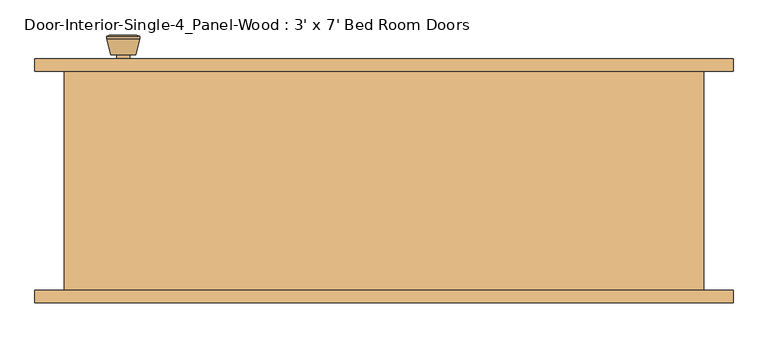
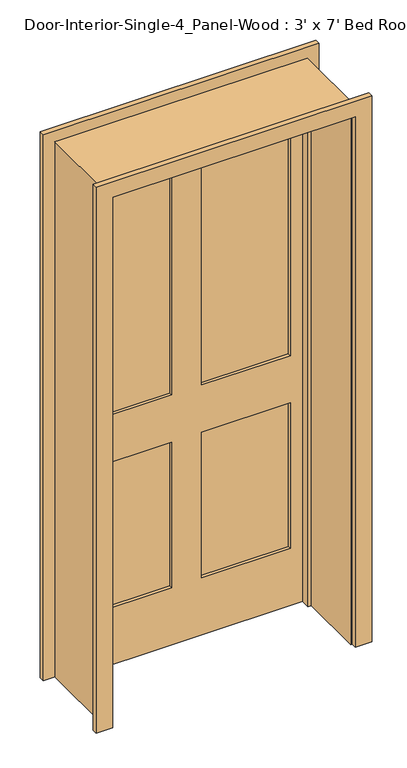
"""IFC4 building model written with IfcOpenShell, lengths in millimetres: door geometry, Door-Interior-Single-4_Panel-Wood : 3' x 7' Bed Room Doors."""

from ifc_helpers import new_model, si_unit, point, frame, frame_2d, origin, place, context, project, spatial, polyline, circle_curve, trimmed, segment, composite_curve, outline, extrude, faceted_brep, source, transform, mapped, element, save
from ifc_brep_helpers import plane_surface, cylinder_surface, revolved_surface, advanced_brep


def door_interior_single_4_panel_wood_3_x_7_bed_room_doors_791c550c(model_context):
    return source(origin(), model_context, "Body", "SolidModel", [
        advanced_brep(
        [(-393.7, 121.0, 914.4), (-383.7, 121.0, 914.4), (-403.7, 121.0, 914.4), (-373.2241324, 72.0, 914.4), (-393.7, 72.0, 914.4), (-414.1758676, 72.0, 914.4), (-368.7, 73.8278681, 914.4), (-418.7, 73.8278681, 914.4), (-368.7, 77.2915463, 914.4), (-418.7, 77.2915463, 914.4), (-375.063764, 102.0, 914.4), (-412.336236, 102.0, 914.4), (-383.7, 102.0, 914.4), (-403.7, 102.0, 914.4)],
        [
            (0, 1),
            (1, 2, circle_curve(frame((-393.7, 121.0, 914.4), z_axis=(0.0, 1.0, 0.0), x_axis=(-1.0, 0.0, 0.0)), 10.0)),
            (2, 0),
            (2, 1, circle_curve(frame((-393.7, 121.0, 914.4), z_axis=(0.0, 1.0, 0.0), x_axis=(-1.0, 0.0, 0.0)), 10.0)),
            (3, 4),
            (4, 5),
            (5, 3, circle_curve(frame((-393.7, 72.0, 914.4), z_axis=(0.0, -1.0, 0.0), x_axis=(-1.0, 0.0, 0.0)), 20.4758676)),
            (3, 5, circle_curve(frame((-393.7, 72.0, 914.4), z_axis=(0.0, -1.0, 0.0), x_axis=(-1.0, 0.0, 0.0)), 20.4758676)),
            (6, 3),
            (5, 7),
            (7, 6, circle_curve(frame((-393.7, 73.8278681, 914.4), z_axis=(0.0, -1.0, 0.0), x_axis=(-1.0, 0.0, 0.0)), 25.0)),
            (6, 7, circle_curve(frame((-393.7, 73.8278681, 914.4), z_axis=(0.0, -1.0, 0.0), x_axis=(-1.0, 0.0, 0.0)), 25.0)),
            (8, 6),
            (7, 9),
            (9, 8, circle_curve(frame((-393.7, 77.2915463, 914.4), z_axis=(0.0, -1.0, 0.0), x_axis=(-1.0, 0.0, 0.0)), 25.0)),
            (8, 9, circle_curve(frame((-393.7, 77.2915463, 914.4), z_axis=(0.0, -1.0, 0.0), x_axis=(-1.0, 0.0, 0.0)), 25.0)),
            (10, 8),
            (9, 11),
            (11, 10, circle_curve(frame((-393.7, 102.0, 914.4), z_axis=(0.0, -1.0, 0.0), x_axis=(-1.0, 0.0, 0.0)), 18.636236)),
            (10, 11, circle_curve(frame((-393.7, 102.0, 914.4), z_axis=(0.0, -1.0, 0.0), x_axis=(-1.0, 0.0, 0.0)), 18.636236)),
            (12, 10),
            (11, 13),
            (13, 12, circle_curve(frame((-393.7, 102.0, 914.4), z_axis=(0.0, -1.0, 0.0), x_axis=(-1.0, 0.0, 0.0)), 10.0)),
            (12, 13, circle_curve(frame((-393.7, 102.0, 914.4), z_axis=(0.0, -1.0, 0.0), x_axis=(-1.0, 0.0, 0.0)), 10.0)),
            (1, 12),
            (13, 2),
        ],
        [
            plane_surface(frame((-393.7, 121.0, 914.4), z_axis=(0.0, 1.0, 0.0), x_axis=(-1.0, 0.0, 0.0))),
            plane_surface(frame((-393.7, 72.0, 914.4), z_axis=(0.0, -1.0, 0.0), x_axis=(-1.0, 0.0, 0.0))),
            revolved_surface(polyline([(-414.1758676, 72.0, 914.4), (-418.7, 73.8278681, 914.4)]), (-393.7, 121.0, 914.4), (0.0, 1.0, 0.0)),
            cylinder_surface(frame((-393.7, 121.0, 914.4), z_axis=(0.0, 1.0, 0.0), x_axis=(-1.0, 0.0, 0.0)), 25.0),
            revolved_surface(polyline([(-418.7, 77.2915463, 914.4), (-412.336236, 102.0, 914.4)]), (-393.7, 121.0, 914.4), (0.0, 1.0, 0.0)),
            plane_surface(frame((-393.7, 102.0, 914.4), z_axis=(0.0, 1.0, 0.0), x_axis=(-1.0, 0.0, 0.0))),
            cylinder_surface(frame((-393.7, 121.0, 914.4), z_axis=(0.0, 1.0, 0.0), x_axis=(-1.0, 0.0, 0.0)), 10.0),
        ],
        [
            (0, [[1, 2, 3]]),
            (0, [[-3, 4, -1]]),
            (1, [[5, 6, 7]]),
            (1, [[-6, -5, 8]]),
            (2, [[9, -7, 10, 11]]),
            (2, [[-10, -8, -9, 12]]),
            (3, [[13, -11, 14, 15]]),
            (3, [[-14, -12, -13, 16]]),
            (4, [[17, -15, 18, 19]]),
            (4, [[-18, -16, -17, 20]]),
            (5, [[21, -19, 22, 23]]),
            (5, [[-22, -20, -21, 24]]),
            (6, [[25, -23, 26, -2]]),
            (6, [[-26, -24, -25, -4]]),
        ],
    ),
        extrude(outline(composite_curve([segment(trimmed(circle_curve(frame_2d((914.4, -393.7)), 30.0), [point((914.4, -423.7))], [point((914.4, -363.7))], False, "CARTESIAN"), True, "CONTINUOUS"), segment(trimmed(circle_curve(frame_2d((914.4, -393.7)), 30.0), [point((914.4, -363.7))], [point((914.4, -423.7))], False, "CARTESIAN"), True, "CONTINUOUS")], self_intersect=False)), frame((0.0, 121.0, 0.0), z_axis=(0.0, 1.0, 0.0), x_axis=(0.0, 0.0, 1.0)), (0.0, 0.0, 1.0), 6.0),
        advanced_brep(
        [(-393.7, 167.925, 914.4), (-403.7, 167.925, 914.4), (-383.7, 167.925, 914.4), (-373.2241324, 216.925, 914.4), (-414.1758676, 216.925, 914.4), (-393.7, 216.925, 914.4), (-368.7, 215.0971319, 914.4), (-418.7, 215.0971319, 914.4), (-368.7, 211.6334537, 914.4), (-418.7, 211.6334537, 914.4), (-375.063764, 186.925, 914.4), (-412.336236, 186.925, 914.4), (-383.7, 186.925, 914.4), (-403.7, 186.925, 914.4)],
        [
            (0, 1),
            (1, 2, circle_curve(frame((-393.7, 167.925, 914.4), z_axis=(0.0, -1.0, 0.0), x_axis=(-1.0, 0.0, 0.0)), 10.0)),
            (2, 0),
            (2, 1, circle_curve(frame((-393.7, 167.925, 914.4), z_axis=(0.0, -1.0, 0.0), x_axis=(-1.0, 0.0, 0.0)), 10.0)),
            (3, 4, circle_curve(frame((-393.7, 216.925, 914.4), z_axis=(0.0, 1.0, 0.0), x_axis=(-1.0, 0.0, 0.0)), 20.4758676)),
            (4, 5),
            (5, 3),
            (4, 3, circle_curve(frame((-393.7, 216.925, 914.4), z_axis=(0.0, 1.0, 0.0), x_axis=(-1.0, 0.0, 0.0)), 20.4758676)),
            (6, 7, circle_curve(frame((-393.7, 215.0971319, 914.4), z_axis=(0.0, 1.0, 0.0), x_axis=(-1.0, 0.0, 0.0)), 25.0)),
            (7, 4),
            (3, 6),
            (7, 6, circle_curve(frame((-393.7, 215.0971319, 914.4), z_axis=(0.0, 1.0, 0.0), x_axis=(-1.0, 0.0, 0.0)), 25.0)),
            (8, 9, circle_curve(frame((-393.7, 211.6334537, 914.4), z_axis=(0.0, 1.0, 0.0), x_axis=(-1.0, 0.0, 0.0)), 25.0)),
            (9, 7),
            (6, 8),
            (9, 8, circle_curve(frame((-393.7, 211.6334537, 914.4), z_axis=(0.0, 1.0, 0.0), x_axis=(-1.0, 0.0, 0.0)), 25.0)),
            (10, 11, circle_curve(frame((-393.7, 186.925, 914.4), z_axis=(0.0, 1.0, 0.0), x_axis=(-1.0, 0.0, 0.0)), 18.636236)),
            (11, 9),
            (8, 10),
            (11, 10, circle_curve(frame((-393.7, 186.925, 914.4), z_axis=(0.0, 1.0, 0.0), x_axis=(-1.0, 0.0, 0.0)), 18.636236)),
            (12, 13, circle_curve(frame((-393.7, 186.925, 914.4), z_axis=(0.0, 1.0, 0.0), x_axis=(-1.0, 0.0, 0.0)), 10.0)),
            (13, 11),
            (10, 12),
            (13, 12, circle_curve(frame((-393.7, 186.925, 914.4), z_axis=(0.0, 1.0, 0.0), x_axis=(-1.0, 0.0, 0.0)), 10.0)),
            (1, 13),
            (12, 2),
        ],
        [
            plane_surface(frame((-393.7, 167.925, 914.4), z_axis=(0.0, -1.0, 0.0), x_axis=(-1.0, 0.0, 0.0))),
            plane_surface(frame((-393.7, 216.925, 914.4), z_axis=(0.0, 1.0, 0.0), x_axis=(-1.0, 0.0, 0.0))),
            revolved_surface(polyline([(-414.1758676, 216.925, 914.4), (-418.7, 215.0971319, 914.4)]), (-393.7, 167.925, 914.4), (0.0, -1.0, 0.0)),
            cylinder_surface(frame((-393.7, 167.925, 914.4), z_axis=(0.0, -1.0, 0.0), x_axis=(-1.0, 0.0, 0.0)), 25.0),
            revolved_surface(polyline([(-418.7, 211.6334537, 914.4), (-412.336236, 186.925, 914.4)]), (-393.7, 167.925, 914.4), (0.0, -1.0, 0.0)),
            plane_surface(frame((-393.7, 186.925, 914.4), z_axis=(0.0, -1.0, 0.0), x_axis=(-1.0, 0.0, 0.0))),
            cylinder_surface(frame((-393.7, 167.925, 914.4), z_axis=(0.0, -1.0, 0.0), x_axis=(-1.0, 0.0, 0.0)), 10.0),
        ],
        [
            (0, [[1, 2, 3]]),
            (0, [[-3, 4, -1]]),
            (1, [[5, 6, 7]]),
            (1, [[8, -7, -6]]),
            (2, [[9, 10, -5, 11]]),
            (2, [[12, -11, -8, -10]]),
            (3, [[13, 14, -9, 15]]),
            (3, [[16, -15, -12, -14]]),
            (4, [[17, 18, -13, 19]]),
            (4, [[20, -19, -16, -18]]),
            (5, [[21, 22, -17, 23]]),
            (5, [[24, -23, -20, -22]]),
            (6, [[-2, 25, -21, 26]]),
            (6, [[-4, -26, -24, -25]]),
        ],
    ),
        extrude(outline(composite_curve([segment(trimmed(circle_curve(frame_2d((914.4, -393.7)), 30.0), [point((914.4, -423.7))], [point((914.4, -363.7))], False, "CARTESIAN"), True, "CONTINUOUS"), segment(trimmed(circle_curve(frame_2d((914.4, -393.7)), 30.0), [point((914.4, -363.7))], [point((914.4, -423.7))], False, "CARTESIAN"), True, "CONTINUOUS")], self_intersect=False)), frame((0.0, 161.925, 0.0), z_axis=(0.0, 1.0, 0.0), x_axis=(0.0, 0.0, 1.0)), (0.0, 0.0, 1.0), 6.0),
        faceted_brep([(482.6, 161.925, 0.0), (482.6, -168.275, 0.0), (457.2, -168.275, 0.0), (457.2, 92.075, 0.0), (444.5, 92.075, 0.0), (444.5, 127.0, 0.0), (457.2, 127.0, 0.0), (457.2, 161.925, 0.0), (482.6, 161.925, 2159.0), (482.6, -168.275, 2159.0), (-482.6, -168.275, 2159.0), (-482.6, -168.275, 0.0), (-457.2, -168.275, 0.0), (-457.2, -168.275, 2133.6), (457.2, -168.275, 2133.6), (457.2, 92.075, 2133.6), (-457.2, 92.075, 2133.6), (-457.2, 92.075, 0.0), (-444.5, 92.075, 0.0), (-444.5, 92.075, 2120.9), (444.5, 92.075, 2120.9), (444.5, 127.0, 2120.9), (-444.5, 127.0, 2120.9), (-444.5, 127.0, 0.0), (-457.2, 127.0, 0.0), (-457.2, 127.0, 2133.6), (457.2, 127.0, 2133.6), (457.2, 161.925, 2133.6), (-457.2, 161.925, 2133.6), (-457.2, 161.925, 0.0), (-482.6, 161.925, 0.0), (-482.6, 161.925, 2159.0)], [[[0, 1, 2, 3, 4, 5, 6, 7]], [[1, 0, 8, 9]], [[2, 1, 9, 10, 11, 12, 13, 14]], [[3, 2, 14, 15]], [[4, 3, 15, 16, 17, 18, 19, 20]], [[5, 4, 20, 21]], [[6, 5, 21, 22, 23, 24, 25, 26]], [[7, 6, 26, 27]], [[0, 7, 27, 28, 29, 30, 31, 8]], [[9, 8, 31, 10]], [[15, 14, 13, 16]], [[21, 20, 19, 22]], [[27, 26, 25, 28]], [[30, 29, 24, 23, 18, 17, 12, 11]], [[10, 31, 30, 11]], [[16, 13, 12, 17]], [[22, 19, 18, 23]], [[28, 25, 24, 29]]]),
        extrude(outline(polyline([(2133.6, -457.2), (0.0, -457.2), (0.0, 457.2), (2133.6, 457.2), (2133.6, -457.2)]), holes=[polyline([(2014.5375, 57.15), (2014.5375, 396.875), (1009.65, 396.875), (1009.65, 57.15), (2014.5375, 57.15)]), polyline([(1009.65, -57.15), (1009.65, -396.875), (2014.5375, -396.875), (2014.5375, -57.15), (1009.65, -57.15)]), polyline([(819.15, 57.15), (819.15, 396.875), (231.775, 396.875), (231.775, 57.15), (819.15, 57.15)]), polyline([(231.775, -57.15), (231.775, -396.875), (819.15, -396.875), (819.15, -57.15), (231.775, -57.15)])]), frame((0.0, 127.0, 0.0), z_axis=(0.0, 1.0, 0.0), x_axis=(0.0, 0.0, 1.0)), (0.0, 0.0, 1.0), 34.925),
        extrude(outline(polyline([(396.875, 138.6416667), (57.15, 138.6416667), (57.15, 150.2833333), (396.875, 150.2833333), (396.875, 138.6416667)])), frame((0.0, 0.0, 1009.65), z_axis=(0.0, 0.0, 1.0), x_axis=(1.0, 0.0, 0.0)), (0.0, 0.0, 1.0), 1004.8875),
        extrude(outline(polyline([(-57.15, 138.6416667), (-396.875, 138.6416667), (-396.875, 150.2833333), (-57.15, 150.2833333), (-57.15, 138.6416667)])), frame((0.0, 0.0, 1009.65), z_axis=(0.0, 0.0, 1.0), x_axis=(1.0, 0.0, 0.0)), (0.0, 0.0, 1.0), 1004.8875),
        extrude(outline(polyline([(396.875, 138.6416667), (57.15, 138.6416667), (57.15, 150.2833333), (396.875, 150.2833333), (396.875, 138.6416667)])), frame((0.0, 0.0, 231.775), z_axis=(0.0, 0.0, 1.0), x_axis=(1.0, 0.0, 0.0)), (0.0, 0.0, 1.0), 587.375),
        extrude(outline(polyline([(-57.15, 138.6416667), (-396.875, 138.6416667), (-396.875, 150.2833333), (-57.15, 150.2833333), (-57.15, 138.6416667)])), frame((0.0, 0.0, 231.775), z_axis=(0.0, 0.0, 1.0), x_axis=(1.0, 0.0, 0.0)), (0.0, 0.0, 1.0), 587.375),
        extrude(outline(polyline([(0.0, 463.55), (0.0, 527.05), (2203.45, 527.05), (2203.45, -527.05), (0.0, -527.05), (0.0, -463.55), (2139.95, -463.55), (2139.95, 463.55), (0.0, 463.55)])), frame((0.0, 161.925, 0.0), z_axis=(0.0, 1.0, 0.0), x_axis=(0.0, 0.0, 1.0)), (0.0, 0.0, 1.0), 19.05),
        extrude(outline(polyline([(0.0, 463.55), (0.0, 527.05), (2203.45, 527.05), (2203.45, -527.05), (0.0, -527.05), (0.0, -463.55), (2139.95, -463.55), (2139.95, 463.55), (0.0, 463.55)])), frame((0.0, -187.325, 0.0), z_axis=(0.0, 1.0, 0.0), x_axis=(0.0, 0.0, 1.0)), (0.0, 0.0, 1.0), 19.05),
    ])


if __name__ == "__main__":
    model = new_model("IFC4")
    model_context = context("Model", 3, world=origin())
    ifc_project = project(units=[si_unit("LENGTHUNIT", "METRE", prefix="MILLI")], contexts=[model_context])
    site = spatial("IfcSite", under=ifc_project)
    building = spatial("IfcBuilding", under=site)
    placement = place(None, origin())
    door_interior_single_4_panel_wood_3_x_7_bed_room_doors_shape = door_interior_single_4_panel_wood_3_x_7_bed_room_doors_791c550c(model_context)
    element("IfcDoor", 1, ObjectType="Door-Interior-Single-4_Panel-Wood : 3' x 7' Bed Room Doors", at=placement, inside=building, context=model_context, shape_type="MappedRepresentation", body=[
        mapped(door_interior_single_4_panel_wood_3_x_7_bed_room_doors_shape, transform((0.0, 0.0, 0.0), x_axis=(1.0, 0.0, 0.0), y_axis=(0.0, 1.0, 0.0), z_axis=(0.0, 0.0, 1.0))),
    ])
    save(model, "model.ifc")

# Revit data of these elements
# Type "Door-Interior-Single-4_Panel-Wood : 3' x 7' Bed Room Doors"
#   Type Mark = "13"
#   Assembly Code = "C1020300"
#   Analytic Construction = "Wooden"
#   Top Rail = 0' - 4 11/16"
#   Thickness = 0' - 1 3/8"
#   Thermal Resistance (R) = 2.5876 (h·ft²·°F)/BTU
#   Swing Angle [instance default] = 90.00°
#   Stiles = 0' - 2 3/8"
#   Rough Width = 3' - 2"
#   Rough Height = 7' - 1"
#   Mullion = 0' - 4 1/2"
#   Lock Rail = 0' - 7 1/2"
#   Height = 7' - 0"
#   Width = 3' - 0"
#   Heat Transfer Coefficient (U) = 0.3865 BTU/(h·ft²·°F)
#   Bottom Rail = 0' - 9 1/8"
#   Trim Material = Cherry
#   Panel Material = Cherry
#   Frame Material = Cherry
#   Door Handle Material = Aluminum
#   Visual Light Transmittance = 0
#   Solar Heat Gain Coefficient = 0
#   Wall Closure = (empty or 0)
#   Function = (empty or 0)
# Element 1 (IfcDoor, "Door-Interior-Single-4_Panel-Wood : 3' x 7' Bed Room Doors")
#   Materials on its faces: "Cherry", "Aluminum"
# Materials
#   "Cherry": class "Wood", colour RGB 226 177 128, transparency 0, Description = "Prunus Serotina", Cost = 0
#   "Aluminum": class "Metal", colour RGB 247 247 247, transparency 0, Description = "Aluminum 6061", Cost = 0
